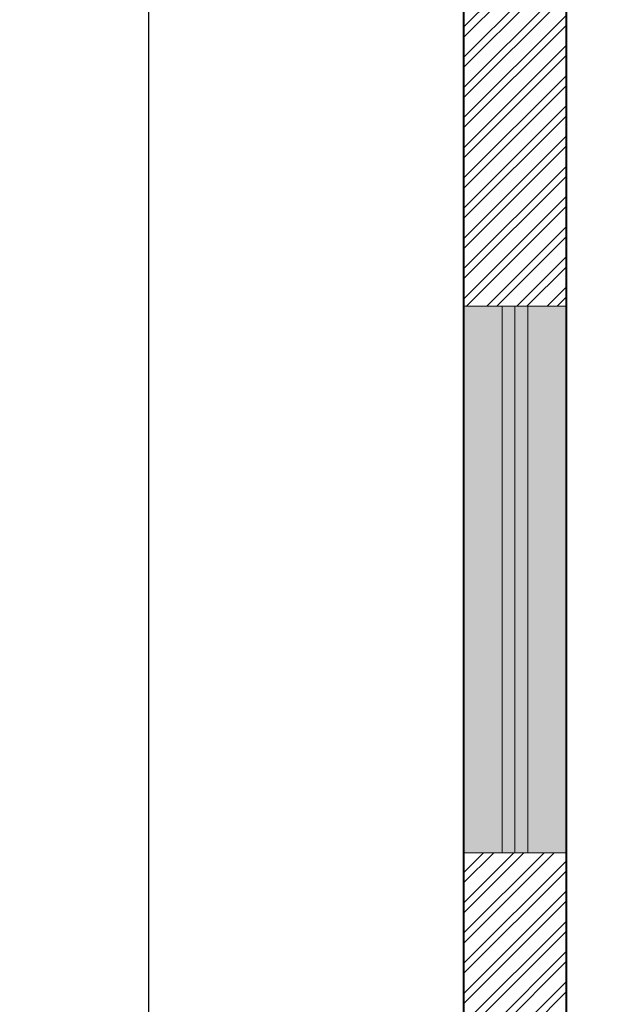
# Model space of a CAD drawing. Units: inches. Extents: x 528 to 2520, y -151 to 1354.
# Tile 31 of 41: x 2119 to 2170, y 731 to 818. Entities that reach past the tile are written whole.
import ezdxf

# ---------------------------------------------------------------- set-up
doc = ezdxf.new("R2010")
doc.units = ezdxf.units.IN
doc.header["$MEASUREMENT"] = 0
for name, color, linetype, lineweight in [('A-ANNO-DIMS', 2, 'Continuous', 18), ('A-ELEV-PROJ', 8, 'Continuous', 13), ('A-WALL-PATT', 6, 'Continuous', 13), ('walls', 7, 'Continuous', 40), ('WINDOWS', 2, 'Continuous', 20)]:
    doc.layers.add(name, color=color, linetype=linetype, lineweight=lineweight)
doc.layers.add('A-GLAZ-PATT', color=152, linetype='Continuous', lineweight=13, true_color=0x2776bb)
doc.styles.get("Standard").update_dxf_attribs({"font": 'arial.ttf'})
doc.dimstyles.get("Standard").update_dxf_attribs({"dimtxt": 6, "dimasz": 2, "dimexe": 0.18, "dimexo": 0.0625, "dimgap": 0.09, "dimtad": 0, "dimtih": 1, "dimtoh": 1, "dimdec": 1, "dimzin": 0, "dimdsep": 46, "dimlunit": 3, "dimtxsty": 'Standard', "dimblk": 'ARCHTICK', "dimcen": 0.09, "dimadec": 0, "dimazin": 0, "dimtfac": 1, "dimtdec": 1, "dimtofl": 0, "dimtmove": 0, "dimatfit": 3, "dimfxl": 1, "dimtolj": 1, "dimtzin": 0, "dimarcsym": 0})

# ---------------------------------------------------------------- blocks, each defined once
blk = doc.blocks.new('WINDOW-48x9-PLAN')
for p, q in [((0, 5.632), (48, 5.632)), ((0, 4.5), (48, 4.5)), ((0, 3.368), (48, 3.368))]:
    blk.add_line(p, q)
blk.add_lwpolyline([(0, 9), (48, 9), (48, 0), (0, 0)], close=True)
blk = doc.blocks.new('_ArchTick')
at = {"color": 0, "linetype": 'ByBlock', "const_width": 0.15}
blk.add_lwpolyline([(-0.5, -0.5), (0.5, 0.5)], dxfattribs=at)
blk = doc.blocks.new('*D95')
at = {"layer": 'A-ANNO-DIMS', "color": 0, "lineweight": -2, "transparency": 16777216}
for p, q in [((2157.95, 897.939), (2130.182, 897.939)), ((2130.362, 897.939), (2130.362, 632.592)), ((2130.362, 360.939), (2130.362, 626.285)), ((2157.95, 360.939), (2130.182, 360.939))]:
    blk.add_line(p, q, dxfattribs=at)
at = {"layer": 'Defpoints', "color": 0, "transparency": 16777216}
for p in [(2130.362, 897.939), (2158.012, 897.939), (2158.012, 360.939)]:
    blk.add_point(p, dxfattribs=at)
at = {"layer": 'A-ANNO-DIMS', "color": 0, "lineweight": -2, "transparency": 16777216, "xscale": 2, "yscale": 2, "zscale": 2}
for p, rotation in [((2130.362, 897.939), 90), ((2130.362, 360.939), 270)]:
    blk.add_blockref('_ArchTick', p, dxfattribs=dict(at, rotation=rotation))
at = {"layer": 'A-ANNO-DIMS', "color": 0, "transparency": 16777216, "insert": (2130.362, 629.439), "char_height": 6, "attachment_point": 5}
blk.add_mtext('\\A1;44\'-9"', dxfattribs=at)

msp = doc.modelspace()

# ---------------------------------------------------------------- hatches: boundary and pattern name
at = {"layer": 'A-GLAZ-PATT'}
h = msp.add_hatch(color=256, dxfattribs=at)
h.dxf.hatch_style = 1
h.paths.add_polyline_path([(2158.012, 792.691), (2158.012, 744.691), (2161.38, 744.691), (2161.38, 792.691)])
h.paths.add_polyline_path([(2161.38, 792.691), (2161.38, 744.691), (2162.512, 744.691), (2162.512, 792.691)])
h.paths.add_polyline_path([(2162.512, 792.691), (2162.512, 744.691), (2163.644, 744.691), (2163.644, 792.691)])
h.paths.add_polyline_path([(2163.644, 792.691), (2163.644, 744.691), (2167.012, 744.691), (2167.012, 792.691)])
at = {"layer": 'A-WALL-PATT'}
h = msp.add_hatch(dxfattribs=at)
h.set_pattern_fill('ANSI32', color=256, scale=5)
h.set_pattern_definition([(45, (1571.3155, -419.1643), (-1.3258252, 1.3258252), []), (45, (1572.1993, -419.1643), (-1.3258252, 1.3258252), [])])
h.paths.add_polyline_path([(2167.012, 744.691), (2158.012, 744.691), (2158.012, 549.939), (2169.559, 549.939), (2174.559, 549.939), (2174.559, 554.939), (2167.012, 554.939), (2167.012, 662.939), (2263.012, 662.939), (2263.012, 667.939), (2263.012, 686.939), (2269.012, 686.939), (2269.012, 691.939), (2258.012, 691.939), (2258.012, 667.939), (2167.012, 667.939)])
h.paths.add_polyline_path([(2260.017, 554.939), (2222.559, 554.939), (2222.559, 549.939), (2260.017, 549.939)])
h.paths.add_polyline_path([(2457.012, 752.205), (2448.012, 752.205), (2448.012, 691.939), (2358.012, 691.939), (2358.012, 686.939), (2448.012, 686.939), (2448.012, 554.939), (2358.012, 554.939), (2358.012, 549.939), (2448.012, 549.939), (2448.012, 405.939), (2406.012, 405.939), (2406.012, 396.939), (2457.012, 396.939)])
h.paths.add_polyline_path([(2457.012, 897.939), (2447.968, 897.939), (2447.968, 888.939), (2448.012, 888.939), (2448.012, 828.939), (2394.012, 828.939), (2394.012, 823.939), (2448.012, 823.939), (2448.012, 800.205), (2457.012, 800.205)])
h.paths.add_polyline_path([(2423.968, 897.939), (2359.012, 897.939), (2359.012, 828.939), (2355.579, 828.939), (2355.579, 823.939), (2364.012, 823.939), (2364.012, 829.939), (2364.012, 888.939), (2423.968, 888.939)])
h.paths.add_polyline_path([(2256.012, 897.939), (2191.012, 897.939), (2191.012, 888.939), (2251.012, 888.939), (2251.012, 828.939), (2251.012, 823.939), (2256.012, 823.939), (2256.012, 829.084)])
h.paths.add_polyline_path([(2167.012, 888.939), (2167.012, 897.939), (2158.012, 897.939), (2158.012, 792.691), (2167.012, 792.691), (2167.012, 823.939), (2221.012, 823.939), (2221.012, 828.939), (2167.012, 828.939)])
h.paths.add_polyline_path([(2316.012, 549.939), (2316.012, 554.939), (2296.017, 554.939), (2296.017, 549.939), (2311.012, 549.939), (2311.012, 455.122), (2316.012, 455.122)])
h.paths.add_polyline_path([(2311.012, 549.939), (2299.012, 549.939), (2299.012, 545.953), (2302.051, 545.953), (2302.051, 542.512), (2305.75, 542.512), (2305.75, 538.075), (2311.012, 538.075)], flags=17)
h.paths.add_polyline_path([(2358.012, 405.939), (2316.012, 405.939), (2316.012, 413.122), (2311.012, 413.122), (2311.012, 396.939), (2358.012, 396.939)])

# ---------------------------------------------------------------- linework, layer by layer
at = {"layer": 'A-ELEV-PROJ'}
msp.add_line((2158.012, 360.939), (2158.012, 897.939), dxfattribs=at)
at = {"layer": 'walls'}
for p, q in [((2158.012, 897.939), (2158.012, 369.939)), ((2167.012, 823.939), (2167.012, 667.939))]:
    msp.add_line(p, q, dxfattribs=at)

# ---------------------------------------------------------------- block references
at = {"layer": 'WINDOWS', "rotation": 90.00000000000044}
msp.add_blockref('WINDOW-48x9-PLAN', (2167.012, 744.691), dxfattribs=at)

# ---------------------------------------------------------------- dimensions: what is measured, and where the dimension line sits
at = {"layer": 'A-ANNO-DIMS'}
dim = msp.add_linear_dim(base=(2130.362, 897.939), p1=(2158.012, 360.939), p2=(2158.012, 897.939), angle=90, dimstyle='Standard', override={"dimdec": 1, "dimlfac": 1, "dimrnd": 0, "dimzin": 1, "dimdsep": 46, "dimlunit": 4, "dimfrac": 2}, dxfattribs=at)
dim.commit()
dim.dimension.update_dxf_attribs({"geometry": '*D95', "text_midpoint": (2130.362, 629.439)})

doc.saveas('drawing.dxf')
